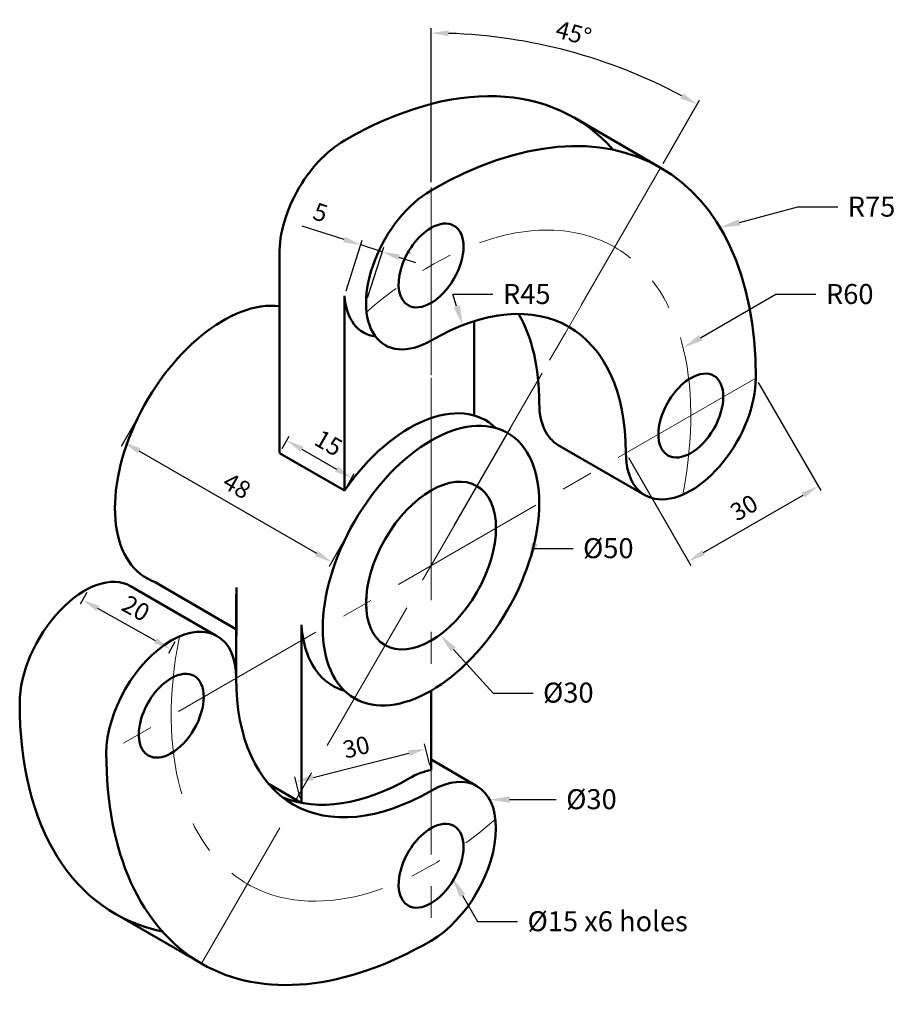
# Model space of a CAD drawing. Units: millimetres. Extents: x 2960 to 3135, y 1692 to 1888.
import ezdxf
from ezdxf import colors
from ezdxf.entities.mleader import LeaderData, LeaderLine
from ezdxf.math import Vec2, Vec3

# ---------------------------------------------------------------- set-up
doc = ezdxf.new("R2010")
doc.units = ezdxf.units.MM
doc.linetypes.add('CENTER', pattern=[50.8, 31.75, -6.35, 6.35, -6.35])
for name, color, linetype, lineweight in [('M-CNTR', 1, 'CENTER', 18), ('M-DIMS', 3, 'Continuous', 25), ('M-OUTL', 7, 'Continuous', 50), ('M-TEXT', 3, 'Continuous', 25)]:
    doc.layers.add(name, color=color, linetype=linetype, lineweight=lineweight)
doc.styles.get("Standard").update_dxf_attribs({"font": 'arial.ttf'})
doc.dimstyles.new('AM_ISO$0', dxfattribs={"dimtxt": 3.5, "dimasz": 3.5, "dimexe": 1, "dimexo": 1, "dimgap": 1.5, "dimtad": 1, "dimdsep": 46, "dimtxsty": 'Standard', "dimcen": 0, "dimclrd": 256, "dimclre": 256, "dimclrt": 2, "dimadec": 0, "dimazin": 2, "dimtp": 0.1, "dimtm": 0.1, "dimtfac": 0.71, "dimtdec": 3, "dimtmove": 0, "dimatfit": 3, "dimfxl": 1, "dimlwd": -1, "dimlwe": -1, "dimarcsym": 1})
doc.dimstyles.new('AM_ISO$2', dxfattribs={"dimtxt": 3.5, "dimasz": 3.5, "dimexe": 1, "dimexo": 1, "dimgap": 1.5, "dimtad": 1, "dimdsep": 46, "dimtxsty": 'Standard', "dimcen": 0, "dimclrd": 256, "dimclre": 256, "dimclrt": 2, "dimadec": 0, "dimazin": 2, "dimtp": 0.1, "dimtm": 0.1, "dimtfac": 0.71, "dimtdec": 3, "dimtmove": 0, "dimatfit": 3, "dimfxl": 1, "dimlwd": -1, "dimlwe": -1, "dimarcsym": 1})

# ---------------------------------------------------------------- blocks, each defined once
blk = doc.blocks.new('*D3')
at = {"layer": 'Defpoints', "color": 0, "transparency": 16777216}
for p in [(3078.97, 1879.36), (3088.49, 1858.87), (3042.56, 1854.95), (3042.56, 1704.32), (2996.64, 1699.77)]:
    blk.add_point(p, dxfattribs=at)
at = {"layer": 'M-DIMS', "color": 0, "linetype": 'ByBlock', "transparency": 16777216}
for p, q in [((3042.56, 1855.95), (3042.56, 1886.78)), ((3088.99, 1859.73), (3096.29, 1872.38))]:
    blk.add_line(p, q, dxfattribs=at)
blk.add_arc((3042.56, 1779.32), 106.46, 61.8838, 88.1162, dxfattribs=at)
at = {"layer": 'M-DIMS', "color": 0, "transparency": 16777216}
for points in [[(3046.05, 1885.14), (3046.07, 1886.3), (3042.56, 1885.78)], [(3093.02, 1873.72), (3092.45, 1872.7), (3095.79, 1871.51)]]:
    blk.add_solid(points, dxfattribs=at)
at = {"layer": 'M-DIMS', "color": 0, "transparency": 16777216, "insert": (3070.97, 1885.32), "char_height": 3.5, "attachment_point": 5, "rotation": 345}
blk.add_mtext('45%%D', dxfattribs=at)
blk = doc.blocks.new('*D4')
at = {"layer": 'Defpoints', "color": 0, "transparency": 16777216}
for p in [(3032.81, 1842.05), (3025.28, 1833.28), (3029.57, 1831.91)]:
    blk.add_point(p, dxfattribs=at)
at = {"layer": 'M-DIMS', "color": 0, "linetype": 'ByBlock', "transparency": 16777216}
for p, q in [((3025.18, 1844.49), (3016.78, 1847.17)), ((3025.58, 1834.23), (3028.82, 1844.38)), ((3032.81, 1842.05), (3028.51, 1843.43)), ((3029.88, 1832.86), (3033.12, 1843.01)), ((3036.15, 1840.99), (3039.48, 1839.92))]:
    blk.add_line(p, q, dxfattribs=at)
at = {"layer": 'M-DIMS', "color": 0, "transparency": 16777216}
for points in [[(3025.36, 1845.05), (3025, 1843.93), (3028.51, 1843.43)], [(3036.32, 1841.54), (3035.97, 1840.43), (3032.81, 1842.05)]]:
    blk.add_solid(points, dxfattribs=at)
at = {"layer": 'M-DIMS', "color": 0, "transparency": 16777216, "insert": (3020.31, 1849.49), "char_height": 3.5, "attachment_point": 5, "rotation": 342.2968}
blk.add_mtext('5', dxfattribs=at)
blk = doc.blocks.new('*D5')
at = {"layer": 'Defpoints', "color": 0, "transparency": 16777216}
for p in [(3012.29, 1801.86), (3026.71, 1796.84), (3025.28, 1794.36)]:
    blk.add_point(p, dxfattribs=at)
at = {"layer": 'M-DIMS', "color": 0, "linetype": 'ByBlock', "transparency": 16777216}
for p, q in [((3012.79, 1802.73), (3014.22, 1805.21)), ((3016.75, 1802.59), (3023.67, 1798.59)), ((3025.78, 1795.23), (3027.21, 1797.71))]:
    blk.add_line(p, q, dxfattribs=at)
at = {"layer": 'M-DIMS', "color": 0, "transparency": 16777216}
for points in [[(3017.04, 1803.1), (3016.46, 1802.09), (3013.72, 1804.34)], [(3023.97, 1799.1), (3023.38, 1798.09), (3026.71, 1796.84)]]:
    blk.add_solid(points, dxfattribs=at)
at = {"layer": 'M-DIMS', "color": 0, "transparency": 16777216, "insert": (3021.85, 1803.44), "char_height": 3.5, "attachment_point": 5, "rotation": 330}
blk.add_mtext('15', dxfattribs=at)
blk = doc.blocks.new('*D6')
at = {"layer": 'Defpoints', "color": 0, "transparency": 16777216}
for p in [(3107.52, 1816.82), (3081.53, 1801.82), (3120.01, 1795.18)]:
    blk.add_point(p, dxfattribs=at)
at = {"layer": 'M-DIMS', "color": 0, "linetype": 'ByBlock', "transparency": 16777216}
for p, q in [((3108.02, 1815.95), (3120.51, 1794.31)), ((3082.03, 1800.95), (3094.53, 1779.31)), ((3097.06, 1781.93), (3116.98, 1793.43))]:
    blk.add_line(p, q, dxfattribs=at)
at = {"layer": 'M-DIMS', "color": 0, "transparency": 16777216}
for points in [[(3116.69, 1793.93), (3117.27, 1792.92), (3120.01, 1795.18)], [(3096.77, 1782.43), (3097.35, 1781.42), (3094.03, 1780.18)]]:
    blk.add_solid(points, dxfattribs=at)
at = {"layer": 'M-DIMS', "color": 0, "transparency": 16777216, "insert": (3105.38, 1790.52), "char_height": 3.5, "attachment_point": 5, "rotation": 30}
blk.add_mtext('30', dxfattribs=at)
blk = doc.blocks.new('*D7')
at = {"layer": 'Defpoints', "color": 0, "transparency": 16777216}
for p in [(2984.22, 1809.44), (3025.79, 1785.44), (3022.67, 1780.03)]:
    blk.add_point(p, dxfattribs=at)
at = {"layer": 'M-DIMS', "color": 0, "linetype": 'ByBlock', "transparency": 16777216}
for p, q in [((2983.72, 1808.57), (2980.6, 1803.16)), ((2984.13, 1802.28), (3019.63, 1781.78)), ((3025.29, 1784.57), (3022.17, 1779.16))]:
    blk.add_line(p, q, dxfattribs=at)
at = {"layer": 'M-DIMS', "color": 0, "transparency": 16777216}
for points in [[(2984.42, 1802.78), (2983.84, 1801.77), (2981.1, 1804.03)], [(3019.93, 1782.28), (3019.34, 1781.27), (3022.67, 1780.03)]]:
    blk.add_solid(points, dxfattribs=at)
at = {"layer": 'M-DIMS', "color": 0, "transparency": 16777216, "insert": (3003.52, 1794.88), "char_height": 3.5, "attachment_point": 5, "rotation": 330}
blk.add_mtext('48', dxfattribs=at)
blk = doc.blocks.new('*D8')
at = {"layer": 'Defpoints', "color": 0, "transparency": 16777216}
for p in [(2974.22, 1774.82), (2972.89, 1772.45), (2991.84, 1764.97)]:
    blk.add_point(p, dxfattribs=at)
at = {"layer": 'M-DIMS', "color": 0, "linetype": 'ByBlock', "transparency": 16777216}
for p, q in [((2973.73, 1773.95), (2972.4, 1771.58)), ((2987.46, 1764.31), (2975.95, 1770.74)), ((2991.35, 1764.09), (2990.03, 1761.72))]:
    blk.add_line(p, q, dxfattribs=at)
at = {"layer": 'M-DIMS', "color": 0, "transparency": 16777216}
for points in [[(2976.23, 1771.25), (2975.66, 1770.23), (2972.89, 1772.45)], [(2987.75, 1764.81), (2987.18, 1763.8), (2990.52, 1762.6)]]:
    blk.add_solid(points, dxfattribs=at)
at = {"layer": 'M-DIMS', "color": 0, "transparency": 16777216, "insert": (2983.31, 1770.39), "char_height": 3.5, "attachment_point": 5, "rotation": 330.7913}
blk.add_mtext('20', dxfattribs=at)
blk = doc.blocks.new('*D9')
at = {"layer": 'Defpoints', "color": 0, "transparency": 16777216}
for p in [(3041.49, 1742.7), (3042.56, 1738.46), (3016.65, 1731.89)]:
    blk.add_point(p, dxfattribs=at)
at = {"layer": 'M-DIMS', "color": 0, "linetype": 'ByBlock', "transparency": 16777216}
for p, q in [((3042.32, 1739.43), (3041.24, 1743.66)), ((3018.96, 1736.98), (3038.1, 1741.84)), ((3016.4, 1732.86), (3015.33, 1737.09))]:
    blk.add_line(p, q, dxfattribs=at)
at = {"layer": 'M-DIMS', "color": 0, "transparency": 16777216}
for points in [[(3037.95, 1742.4), (3038.24, 1741.27), (3041.49, 1742.7)], [(3018.82, 1737.55), (3019.11, 1736.42), (3015.57, 1736.12)]]:
    blk.add_solid(points, dxfattribs=at)
at = {"layer": 'M-DIMS', "color": 0, "transparency": 16777216, "insert": (3027.72, 1742.6), "char_height": 3.5, "attachment_point": 5, "rotation": 14.2257}
blk.add_mtext('30', dxfattribs=at)

msp = doc.modelspace()

# ---------------------------------------------------------------- linework, layer by layer
at = {"layer": 'M-CNTR'}
for p, q in [((3088.491, 1858.868), (2996.636, 1699.769)), ((3042.563, 1779.318), (3088.491, 1858.868)), ((3042.563, 1779.318), (3042.563, 1854.952)), ((3042.563, 1854.952), (3042.563, 1704.318)), ((3107.515, 1816.818), (2977.612, 1741.818))]:
    msp.add_line(p, q, dxfattribs=at)
for start_param, end_param in [(2.1055388, 4.1776465), (5.2471315, 7.3192391)]:
    msp.add_ellipse((3042.563, 1779.318), major_axis=(-36.742, -63.64), ratio=0.5773503, start_param=start_param, end_param=end_param, dxfattribs=at)
at = {"layer": 'M-OUTL'}
for p, q in [((3071.171, 1868.868), (3088.491, 1858.868)), ((3012.285, 1840.778), (3012.285, 1801.865)), ((3038.277, 1841.793), (3038.233, 1841.818)), ((3025.275, 1833.278), (3025.275, 1794.365)), ((3051.224, 1809.318), (3051.224, 1828.193)), ((3068.019, 1803.408), (3085.339, 1793.408)), ((3025.243, 1794.318), (3012.253, 1801.818)), ((3003.655, 1766.538), (2987.419, 1776.005)), ((2999.522, 1765.373), (2982.467, 1775.228)), ((3003.592, 1756.818), (3003.592, 1773.543)), ((3003.655, 1774.957), (3003.655, 1765.289)), ((3029.606, 1772.896), (3029.606, 1770.778)), ((3003.592, 1767.042), (3003.655, 1767.004)), ((3016.645, 1767.457), (3016.645, 1731.89)), ((3022.537, 1755.537), (3022.924, 1755.302)), ((3022.924, 1755.302), (3022.848, 1755.346)), ((3042.563, 1754.318), (3042.563, 1738.46)), ((3042.563, 1740.531), (3051.749, 1735.228)), ((3010.16, 1735.61), (3016.583, 1731.902)), ((2979.315, 1709.769), (2996.636, 1699.769))]:
    msp.add_line(p, q, dxfattribs=at)
for centre, major_axis, start_param, end_param in [((3025.243, 1789.318), (-45.928, -79.55), 9.2350805, 10.2101761), ((3042.563, 1779.318), (-45.928, -79.55), 8.6393798, 10.2101761), ((3025.243, 1849.318), (-9.186, -15.91), 3.9269908, 5.5684433), ((3042.563, 1839.318), (-9.186, -15.91), 3.9269908, 7.0685835), ((3042.563, 1839.318), (4.593, 7.955), 0.7853982, 3.1415927), ((3042.563, 1839.318), (4.593, 7.955), 3.1415927, 6.2831853), ((3042.563, 1839.318), (4.593, 7.955), 0, 0.7853982), ((3038.233, 1841.818), (-9.186, -15.91), 5.5684433, 6.5211264), ((3000.994, 1803.318), (-15.309, -26.517), 3.3783863, 6.3908953), ((3042.563, 1779.318), (-27.557, -47.73), 8.6393798, 10.2101761), ((3025.243, 1789.318), (-27.557, -47.73), 8.6393798, 9.1050907), ((3094.525, 1809.318), (-9.186, -15.91), 5.4977871, 8.6393798), ((3094.525, 1809.318), (4.593, 7.955), 0.7853982, 3.1415927), ((3094.525, 1809.318), (4.593, 7.955), 3.1415927, 6.2831853), ((3094.525, 1809.318), (4.593, 7.955), 0, 0.7853982), ((3038.233, 1781.818), (-15.309, -26.517), 2.9996956, 4.5686219), ((3077.205, 1819.318), (-9.186, -15.91), 5.4977871, 6.2831853), ((2973.281, 1759.318), (-9.186, -15.91), 3.1411566, 5.4977871), ((2990.602, 1749.318), (-9.186, -15.91), 2.3561945, 5.4977871), ((3038.233, 1781.818), (-15.309, -26.517), 5.5737302, 6.2575609), ((2990.602, 1749.318), (4.593, 7.955), 0, 0.7853982), ((2990.602, 1749.318), (4.593, 7.955), 0.7853982, 3.1415927), ((2990.602, 1749.318), (4.593, 7.955), 3.1415927, 6.2831853), ((3042.563, 1779.318), (-27.557, -47.73), 5.4977871, 7.0685835), ((3038.233, 1781.818), (-15.309, -26.517), 6.2782002, 6.4250824), ((3025.243, 1789.318), (-45.928, -79.55), 5.4977871, 6.4728828), ((3042.563, 1779.318), (-45.928, -79.55), 5.4977871, 7.0685835), ((3038.233, 1721.818), (-9.186, -15.91), 3.5871539, 3.9269908), ((3042.563, 1719.318), (-9.186, -15.91), 7.0685835, 10.2101761), ((3038.233, 1781.818), (-27.557, -47.73), 6.3618338, 7.0685835), ((3042.563, 1719.318), (4.593, 7.955), 0.7853982, 3.1415927), ((3042.563, 1719.318), (4.593, 7.955), 3.1415927, 6.2831853), ((3042.563, 1719.318), (4.593, 7.955), 0, 0.7853982)]:
    msp.add_ellipse(centre, major_axis=major_axis, ratio=0.5773503, start_param=start_param, end_param=end_param, dxfattribs=at)
for major_axis in [(-15.309, -26.517), (-9.186, -15.91)]:
    msp.add_ellipse((3042.563, 1779.318), major_axis=major_axis, ratio=0.5773503, dxfattribs=at)

# ---------------------------------------------------------------- dimensions: what is measured, and where the dimension line sits
at = {"layer": 'M-DIMS'}
dim = msp.add_angular_dim_2l(base=(3078.975, 1879.357), line1=((3042.563, 1854.952), (3042.563, 1704.318)), line2=((3088.491, 1858.868), (2996.636, 1699.769)), text='45%%D', dimstyle='AM_ISO$2', override={"dimpost": '', "dimclrd": 0, "dimclre": 0, "dimclrt": 0}, dxfattribs=at)
dim.commit()
dim.dimension.update_dxf_attribs({"geometry": '*D3', "text_midpoint": (3070.966, 1885.318)})
dim = msp.add_linear_dim(base=(3032.812, 1842.053), p1=(3025.275, 1833.278), p2=(3029.573, 1831.906), angle=342.29677, text='5', dimstyle='AM_ISO$0', override={"dimclrd": 0, "dimclre": 0, "dimclrt": 0}, dxfattribs=at)
dim.commit()
dim.dimension.update_dxf_attribs({"geometry": '*D4', "text_midpoint": (3019.312, 1846.363), "dimtype": 161})
for p1, p2, distance, override, picture, middle in [((3081.535, 1801.818), (3107.515, 1816.818), -24.99, {"dimclrd": 0, "dimclre": 0, "dimclrt": 0}, '*D6', (3105.376, 1790.524)), ((2984.22, 1809.44), (3025.79, 1785.44), -6.249, {"dimclrd": 0, "dimclre": 0, "dimclrt": 0}, '*D7', (3003.524, 1794.876)), ((3012.285, 1801.865), (3025.275, 1794.365), 2.861, {"dimpost": '', "dimclrd": 0, "dimclre": 0, "dimclrt": 0}, '*D5', (3021.854, 1803.439))]:
    dim = msp.add_aligned_dim(p1=p1, p2=p2, distance=distance, dimstyle='AM_ISO$0', override=override, dxfattribs=at)
    dim.commit()
    dim.dimension.update_dxf_attribs({"geometry": picture, "text_midpoint": middle})
for p1, p2, distance, text, picture, middle in [((2991.842, 1764.965), (2974.217, 1774.819), 2.713, '20', '*D8', (2983.309, 1770.394)), ((3016.645, 1731.89), (3042.563, 1738.46), 4.369, '30', '*D9', (3027.723, 1742.597))]:
    dim = msp.add_aligned_dim(p1=p1, p2=p2, distance=distance, text=text, dimstyle='AM_ISO$0', override={"dimpost": '', "dimclrd": 0, "dimclre": 0, "dimclrt": 0}, dxfattribs=at)
    dim.commit()
    dim.dimension.update_dxf_attribs({"geometry": picture, "text_midpoint": middle})

# ---------------------------------------------------------------- leaders
at = {"layer": 'M-TEXT'}
ml = msp.add_multileader_mtext('Standard', dxfattribs=at)
ml.set_content('{\\C2;R75}', color=256)
ml.set_leader_properties()
ml.build(insert=Vec2(0, 0))
ctx = ml.context
ctx.base_point, ctx.plane_origin = Vec3(3123.901, 1851.047), Vec3(3100.368, 1846.894)
notes = []
notes.append((ctx, [(0, (1, 1, 0), (3115.901, 1851.047), (1, 0), 8, [(0, [(3100.368, 1846.894)], 0, [])])]))
ctx.mtext.insert, ctx.mtext.flow_direction = Vec3(3125.901, 1853.082), 5
ml = msp.add_multileader_mtext('Standard', dxfattribs=at)
ml.set_content('{\\C2;R45}', color=256)
ml.set_leader_properties()
ml.build(insert=Vec2(0, 0))
ctx = ml.context
ctx.base_point, ctx.plane_origin = Vec3(3054.944, 1833.583), Vec3(3048.88, 1827.37)
notes.append((ctx, [(0, (1, 1, 0), (3046.944, 1833.583), (1, 0), 8, [(0, [(3048.88, 1827.37)], 0, [])])]))
ctx.mtext.insert, ctx.mtext.flow_direction = Vec3(3056.944, 1835.618), 5
ml = msp.add_multileader_mtext('Standard', dxfattribs=at)
ml.set_content('{\\C2;R60}', color=256)
ml.set_leader_properties()
ml.build(insert=Vec2(0, 0))
ctx = ml.context
ctx.base_point, ctx.plane_origin = Vec3(3119.541, 1833.579), Vec3(3092.999, 1822.873)
notes.append((ctx, [(0, (1, 1, 0), (3111.541, 1833.579), (1, 0), 8, [(0, [(3092.999, 1822.873)], 0, [])])]))
ctx.mtext.insert, ctx.mtext.flow_direction = Vec3(3121.541, 1835.613), 5
ml = msp.add_multileader_mtext('Standard', dxfattribs=at)
ml.set_content('{\\C2;%%C50}', color=256)
ml.set_leader_properties()
ml.build(insert=Vec2(0, 0))
ctx = ml.context
ctx.base_point, ctx.plane_origin = Vec3(3070.965, 1782.728), Vec3(3062.129, 1779.911)
notes.append((ctx, [(0, (1, 1, 0), (3062.965, 1782.728), (1, 0), 8, [(0, [(3062.129, 1779.911)], 0, [])])]))
ctx.mtext.insert, ctx.mtext.flow_direction = Vec3(3072.965, 1784.808), 5
ml = msp.add_multileader_mtext('Standard', dxfattribs=at)
ml.set_content('{\\C2;%%C30}', color=256)
ml.set_leader_properties()
ml.build(insert=Vec2(0, 0))
ctx = ml.context
ctx.base_point, ctx.plane_origin = Vec3(3062.969, 1753.849), Vec3(3044.349, 1765.491)
notes.append((ctx, [(0, (1, 1, 0), (3054.969, 1753.849), (1, 0), 8, [(0, [(3044.349, 1765.491)], 0, [])])]))
ctx.mtext.insert, ctx.mtext.flow_direction = Vec3(3064.969, 1755.93), 5
ml = msp.add_multileader_mtext('Standard', dxfattribs=at)
ml.set_content('{\\C2;%%C30}', color=256)
ml.set_leader_properties()
ml.build(insert=Vec2(0, 0))
ctx = ml.context
ctx.base_point, ctx.plane_origin = Vec3(3067.594, 1732.545), Vec3(3054.288, 1732.545)
notes.append((ctx, [(0, (1, 1, 0), (3059.594, 1732.545), (1, 0), 8, [(0, [(3054.288, 1732.545)], 0, [])])]))
ctx.mtext.insert, ctx.mtext.flow_direction = Vec3(3069.594, 1734.626), 5
ml = msp.add_multileader_mtext('Standard', dxfattribs=at)
ml.set_content('{\\C2;%%C15 x6 holes}', color=256)
ml.set_leader_properties()
ml.build(insert=Vec2(0, 0))
ctx = ml.context
ctx.base_point, ctx.plane_origin = Vec3(3059.868, 1708.152), Vec3(3046.85, 1716.843)
notes.append((ctx, [(0, (1, 1, 0), (3051.868, 1708.152), (1, 0), 8, [(0, [(3046.85, 1716.843)], 0, [])])]))
ctx.mtext.insert, ctx.mtext.flow_direction = Vec3(3061.868, 1710.233), 5
for ctx, leaders in notes:
    for number, flags, end, landing, length, lines in leaders:
        leader = LeaderData()
        leader.index, (leader.has_last_leader_line, leader.has_dogleg_vector, leader.attachment_direction) = number, flags
        leader.last_leader_point, leader.dogleg_vector, leader.dogleg_length = Vec3(end), Vec3(landing), length
        for number, points, colour, breaks in lines:
            line = LeaderLine()
            line.index, line.vertices, line.color, line.breaks = number, Vec3.list(points), colors.encode_raw_color(colour), breaks
            leader.lines.append(line)
        ctx.leaders.append(leader)

doc.saveas('drawing.dxf')
